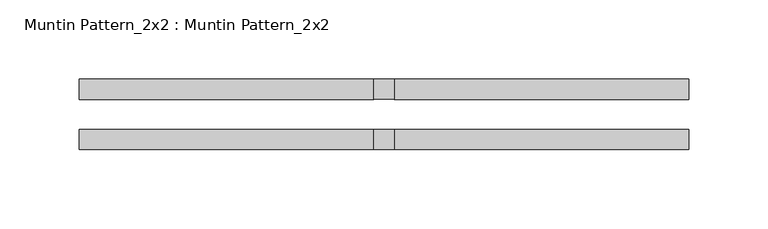
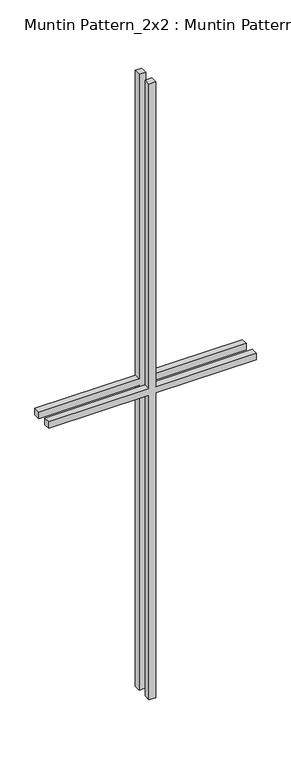
"""IFC4 building model written with IfcOpenShell, lengths in millimetres: proxy geometry, Muntin Pattern_2x2 : Muntin Pattern_2x2."""

from ifc_helpers import new_model, si_unit, frame, origin, place, context, project, spatial, polyline, outline, extrude, source, transform, mapped, element, save


def muntin_pattern_2x2_muntin_pattern_2x2_3dfd0a47(model_context):
    return source(origin(), model_context, "Body", "SweptSolid", [
        extrude(outline(polyline([(609.6, -6.35), (609.6, -192.0875), (596.9, -192.0875), (596.9, -6.35), (0.0, -6.35), (0.0, 6.35), (596.9, 6.35), (596.9, 192.0875), (609.6, 192.0875), (609.6, 6.35), (1206.5, 6.35), (1206.5, -6.35), (609.6, -6.35)])), frame((0.0, -22.225, 0.0), z_axis=(0.0, 1.0, 0.0), x_axis=(0.0, 0.0, 1.0)), (0.0, 0.0, 1.0), 12.7),
        extrude(outline(polyline([(609.6, -6.35), (609.6, -192.0875), (596.9, -192.0875), (596.9, -6.35), (0.0, -6.35), (0.0, 6.35), (596.9, 6.35), (596.9, 192.0875), (609.6, 192.0875), (609.6, 6.35), (1206.5, 6.35), (1206.5, -6.35), (609.6, -6.35)])), frame((0.0, 9.525, 0.0), z_axis=(0.0, 1.0, 0.0), x_axis=(0.0, 0.0, 1.0)), (0.0, 0.0, 1.0), 12.7),
    ])


if __name__ == "__main__":
    model = new_model("IFC4")
    model_context = context("Model", 3, world=origin())
    ifc_project = project(units=[si_unit("LENGTHUNIT", "METRE", prefix="MILLI")], contexts=[model_context])
    site = spatial("IfcSite", under=ifc_project)
    building = spatial("IfcBuilding", under=site)
    placement = place(None, origin())
    muntin_pattern_2x2_muntin_pattern_2x2_shape = muntin_pattern_2x2_muntin_pattern_2x2_3dfd0a47(model_context)
    element("IfcBuildingElementProxy", 1, Name="Muntin Pattern_2x2 : Muntin Pattern_2x2", ObjectType="Muntin Pattern_2x2 : Muntin Pattern_2x2", at=placement, inside=building, context=model_context, shape_type="MappedRepresentation", body=[
        mapped(muntin_pattern_2x2_muntin_pattern_2x2_shape, transform((0.0, 0.0, 0.0), x_axis=(1.0, 0.0, 0.0), y_axis=(0.0, 1.0, 0.0), z_axis=(0.0, 0.0, 1.0))),
    ])
    save(model, "model.ifc")

# Revit data of these elements
# Type "Muntin Pattern_2x2 : Muntin Pattern_2x2"
#   Width [instance default] = 4' - 0"
#   Thickness = 0' - 0 1/2"
#   Height [instance default] = 4' - 0"
#   Distance = 0' - 0 3/4"
#   Interior Material [instance default] = none
#   Exterior Material [instance default] = none
#   Default Elevation = 0
# Element 1 (IfcBuildingElementProxy, "Muntin Pattern_2x2 : Muntin Pattern_2x2")
#   Width = 1' - 3 1/8"
#   Height = 3' - 11 1/2"
#   Interior Material = Wood - Stained
#   Exterior Material = Clad - White
#   Materials on its faces: "Clad - White", "Wood - Stained"
# Materials
#   "Clad - White": class "Wood", colour RGB 30 30 30, transparency 0, Cost = 0
#   "Wood - Stained": class "Wood", colour RGB 224 178 126, transparency 0, Cost = 0
